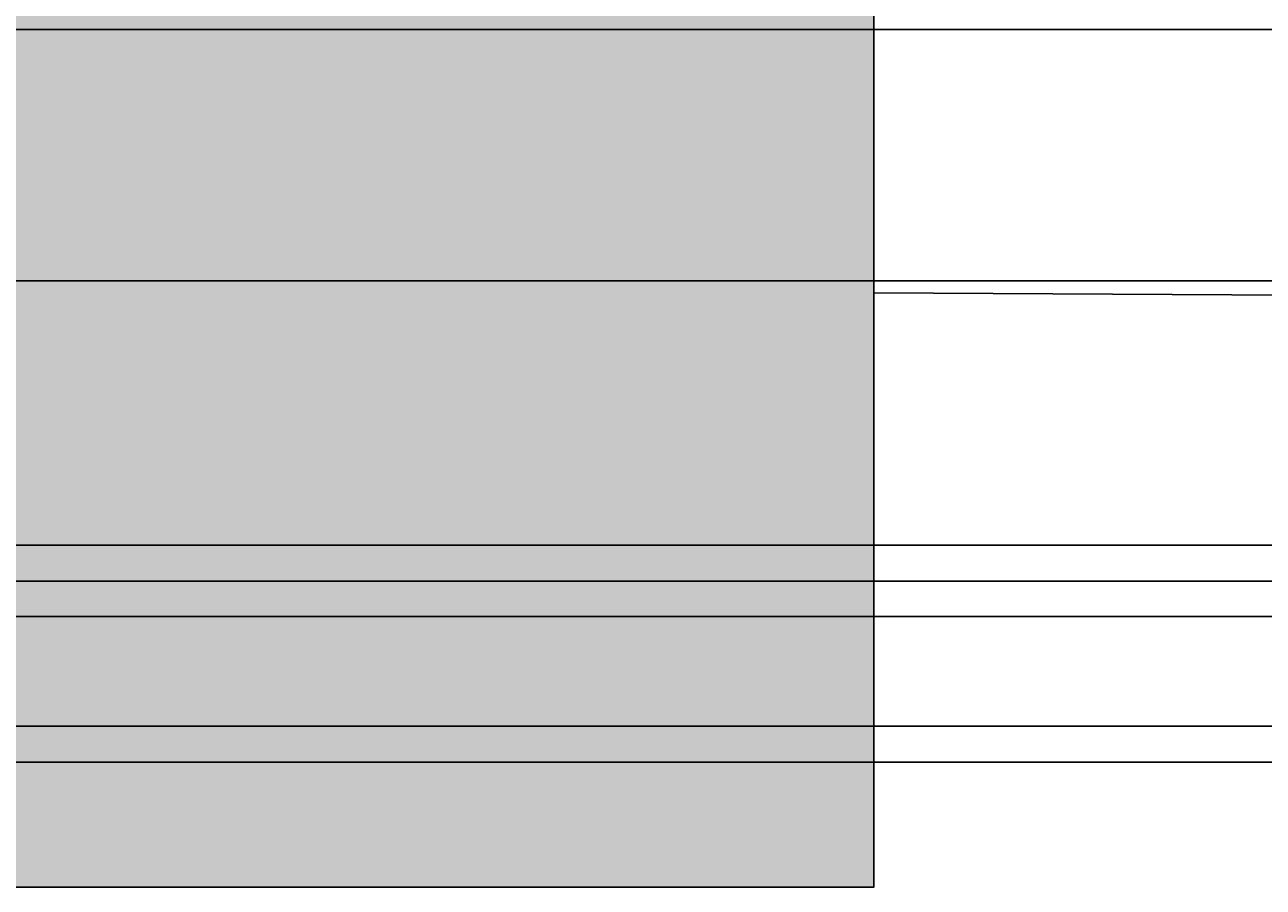
# Model space of a CAD drawing. Units: inches. Extents: x 35362 to 73946, y 43607 to 67532.
# Tile 5 of 134: x 37937 to 40793, y 46919 to 48909. Entities that reach past the tile are written whole.
import ezdxf

# ---------------------------------------------------------------- set-up
doc = ezdxf.new("R2010")
doc.units = ezdxf.units.IN
doc.header["$MEASUREMENT"] = 0
for name, color, linetype, lineweight in [('A-ANNO-DIMS', 2, 'Continuous', 18), ('E-SYMB', 1, 'Continuous', 25), ('E-SYMB-PATT', 1, 'Continuous', 13), ('E-WIRE', 3, 'Continuous', 25)]:
    doc.layers.add(name, color=color, linetype=linetype, lineweight=lineweight)
doc.styles.get("Standard").update_dxf_attribs({"font": 'arial.ttf'})
doc.dimstyles.get("Standard").update_dxf_attribs({"dimtxt": 0.18, "dimasz": 0.18, "dimexe": 0.18, "dimexo": 0.0625, "dimgap": 0.09, "dimtad": 0, "dimtih": 1, "dimtoh": 1, "dimdec": 4, "dimzin": 0, "dimdsep": 46, "dimtxsty": 'Standard', "dimcen": 0.09, "dimadec": 0, "dimazin": 0, "dimtfac": 1, "dimtdec": 4, "dimtofl": 0, "dimtmove": 0, "dimatfit": 3, "dimfxl": 1, "dimtolj": 1, "dimtzin": 0, "dimarcsym": 0})

# ---------------------------------------------------------------- blocks, each defined once
blk = doc.blocks.new('*D43')
at = {"layer": 'A-ANNO-DIMS', "color": 0, "lineweight": -2, "transparency": 16777216}
for p, q in [((62004.7, 47625.2), (35361.8, 47625.2)), ((35361.9, 47625), (35361.9, 47416.9)), ((35361.9, 47208.4), (35361.9, 47416.5)), ((62004.7, 47208.2), (35361.8, 47208.2))]:
    blk.add_line(p, q, dxfattribs=at)
at = {"layer": 'A-ANNO-DIMS', "color": 0, "transparency": 16777216}
for points in [[(35361.9, 47625), (35362, 47625), (35361.9, 47625.2)], [(35361.9, 47208.4), (35362, 47208.4), (35361.9, 47208.2)]]:
    blk.add_solid(points, dxfattribs=at)
at = {"layer": 'Defpoints', "color": 0, "transparency": 16777216}
for p in [(62004.7, 47625.2), (35361.9, 47208.2), (62004.7, 47208.2)]:
    blk.add_point(p, dxfattribs=at)
at = {"layer": 'A-ANNO-DIMS', "color": 0, "transparency": 16777216, "insert": (35361.9, 47416.7), "char_height": 0.18, "attachment_point": 5}
blk.add_mtext('\\A1;416.9', dxfattribs=at)
blk = doc.blocks.new('*D67')
at = {"layer": 'A-ANNO-DIMS', "color": 0, "lineweight": -2, "transparency": 16777216}
for p, q in [((56873.5, 53351.5), (35361.8, 53351.5)), ((35361.9, 53351.3), (35361.9, 49400.9)), ((35361.9, 45450.1), (35361.9, 49400.5)), ((53793.6, 45449.9), (35361.8, 45449.9))]:
    blk.add_line(p, q, dxfattribs=at)
at = {"layer": 'A-ANNO-DIMS', "color": 0, "transparency": 16777216}
for points in [[(35361.9, 53351.3), (35362, 53351.3), (35361.9, 53351.5)], [(35361.9, 45450.1), (35362, 45450.1), (35361.9, 45449.9)]]:
    blk.add_solid(points, dxfattribs=at)
at = {"layer": 'Defpoints', "color": 0, "transparency": 16777216}
for p in [(35361.9, 53351.5), (56873.6, 53351.5), (53793.6, 45449.9)]:
    blk.add_point(p, dxfattribs=at)
at = {"layer": 'A-ANNO-DIMS', "color": 0, "transparency": 16777216, "insert": (35361.9, 49400.7), "char_height": 0.18, "attachment_point": 5}
blk.add_mtext('\\A1;7901.6', dxfattribs=at)
blk = doc.blocks.new('*D87')
at = {"layer": 'A-ANNO-DIMS', "color": 0, "lineweight": -2, "transparency": 16777216}
for p, q in [((52362.5, 48318.3), (35361.8, 48318.3)), ((35361.9, 48318.1), (35361.9, 47931.4)), ((35361.9, 47544.3), (35361.9, 47931)), ((52362.5, 47544.1), (35361.8, 47544.1))]:
    blk.add_line(p, q, dxfattribs=at)
at = {"layer": 'A-ANNO-DIMS', "color": 0, "transparency": 16777216}
for points in [[(35361.9, 48318.1), (35362, 48318.1), (35361.9, 48318.3)], [(35361.9, 47544.3), (35362, 47544.3), (35361.9, 47544.1)]]:
    blk.add_solid(points, dxfattribs=at)
at = {"layer": 'Defpoints', "color": 0, "transparency": 16777216}
for p in [(35361.9, 48318.3), (52362.6, 48318.3), (52362.6, 47544.1)]:
    blk.add_point(p, dxfattribs=at)
at = {"layer": 'A-ANNO-DIMS', "color": 0, "transparency": 16777216, "insert": (35361.9, 47931.2), "char_height": 0.18, "attachment_point": 5}
blk.add_mtext('\\A1;774.1', dxfattribs=at)
blk = doc.blocks.new('*D89')
at = {"layer": 'A-ANNO-DIMS', "color": 0, "lineweight": -2, "transparency": 16777216}
for p, q in [((53707.7, 48897.7), (35361.8, 48897.7)), ((35361.9, 48897.6), (35361.9, 48303.2)), ((35361.9, 47708.4), (35361.9, 48302.8)), ((53707.7, 47708.2), (35361.8, 47708.2))]:
    blk.add_line(p, q, dxfattribs=at)
at = {"layer": 'A-ANNO-DIMS', "color": 0, "transparency": 16777216}
for points in [[(35361.9, 48897.6), (35362, 48897.6), (35361.9, 48897.7)], [(35361.9, 47708.4), (35362, 47708.4), (35361.9, 47708.2)]]:
    blk.add_solid(points, dxfattribs=at)
at = {"layer": 'Defpoints', "color": 0, "transparency": 16777216}
for p in [(53707.8, 48897.7), (35361.9, 47708.2), (53707.8, 47708.2)]:
    blk.add_point(p, dxfattribs=at)
at = {"layer": 'A-ANNO-DIMS', "color": 0, "transparency": 16777216, "insert": (35361.9, 48303), "char_height": 0.18, "attachment_point": 5}
blk.add_mtext('\\A1;1189.5', dxfattribs=at)
blk = doc.blocks.new('*D90')
at = {"layer": 'A-ANNO-DIMS', "color": 0, "lineweight": -2, "transparency": 16777216}
for p, q in [((53707.7, 47291.3), (35361.8, 47291.3)), ((35361.9, 47291.1), (35361.9, 46710.3)), ((35361.9, 46129.1), (35361.9, 46709.9)), ((53793.6, 46128.9), (35361.8, 46128.9))]:
    blk.add_line(p, q, dxfattribs=at)
at = {"layer": 'A-ANNO-DIMS', "color": 0, "transparency": 16777216}
for points in [[(35361.9, 47291.1), (35362, 47291.1), (35361.9, 47291.3)], [(35361.9, 46129.1), (35362, 46129.1), (35361.9, 46128.9)]]:
    blk.add_solid(points, dxfattribs=at)
at = {"layer": 'Defpoints', "color": 0, "transparency": 16777216}
for p in [(53707.8, 47291.3), (35361.9, 46128.9), (53793.6, 46128.9)]:
    blk.add_point(p, dxfattribs=at)
at = {"layer": 'A-ANNO-DIMS', "color": 0, "transparency": 16777216, "insert": (35361.9, 46710.1), "char_height": 0.18, "attachment_point": 5}
blk.add_mtext('\\A1;1162.4', dxfattribs=at)

msp = doc.modelspace()

# ---------------------------------------------------------------- hatches: boundary and pattern name
at = {"layer": 'E-SYMB-PATT'}
h = msp.add_hatch(color=256, dxfattribs=at)
h.dxf.hatch_style = 1
h.paths.add_polyline_path([(39894.84, 49689.843), (37121.949, 49689.843), (37121.949, 46919.381), (39894.84, 46919.381)])

# ---------------------------------------------------------------- linework, layer by layer
at = {"layer": 'E-SYMB'}
msp.add_lwpolyline([(37121.949, 49689.843), (39894.84, 49689.843), (39894.84, 46919.381), (37121.949, 46919.381)], close=True, dxfattribs=at)
at = {"layer": 'E-WIRE'}
msp.add_line((39894.84, 48290.562), (42056.036, 48277.555), dxfattribs=at)

# ---------------------------------------------------------------- dimensions: what is measured, and where the dimension line sits
at = {"layer": 'A-ANNO-DIMS'}
for base, p1, p2, picture, middle in [((35361.949, 53351.529), (53793.638, 45449.894), (56873.602, 53351.529), '*D67', (35361.949, 49400.712)), ((35361.949, 47708.216), (53707.781, 48897.738), (53707.781, 47708.216), '*D89', (35361.949, 48302.977)), ((35361.949, 48318.269), (52362.557, 47544.134), (52362.557, 48318.269), '*D87', (35361.949, 47931.201)), ((35361.949, 47208.25), (62004.728, 47625.181), (62004.728, 47208.25), '*D43', (35361.949, 47416.715)), ((35361.949, 46128.878), (53707.781, 47291.285), (53793.638, 46128.878), '*D90', (35361.949, 46710.081))]:
    dim = msp.add_linear_dim(base=base, p1=p1, p2=p2, angle=90, dimstyle='Standard', override={"dimdec": 1, "dimlfac": 1, "dimrnd": 0, "dimzin": 0, "dimdsep": 46, "dimlunit": 2}, dxfattribs=at)
    dim.commit()
    dim.dimension.update_dxf_attribs({"geometry": picture, "text_midpoint": middle})

doc.saveas('drawing.dxf')
